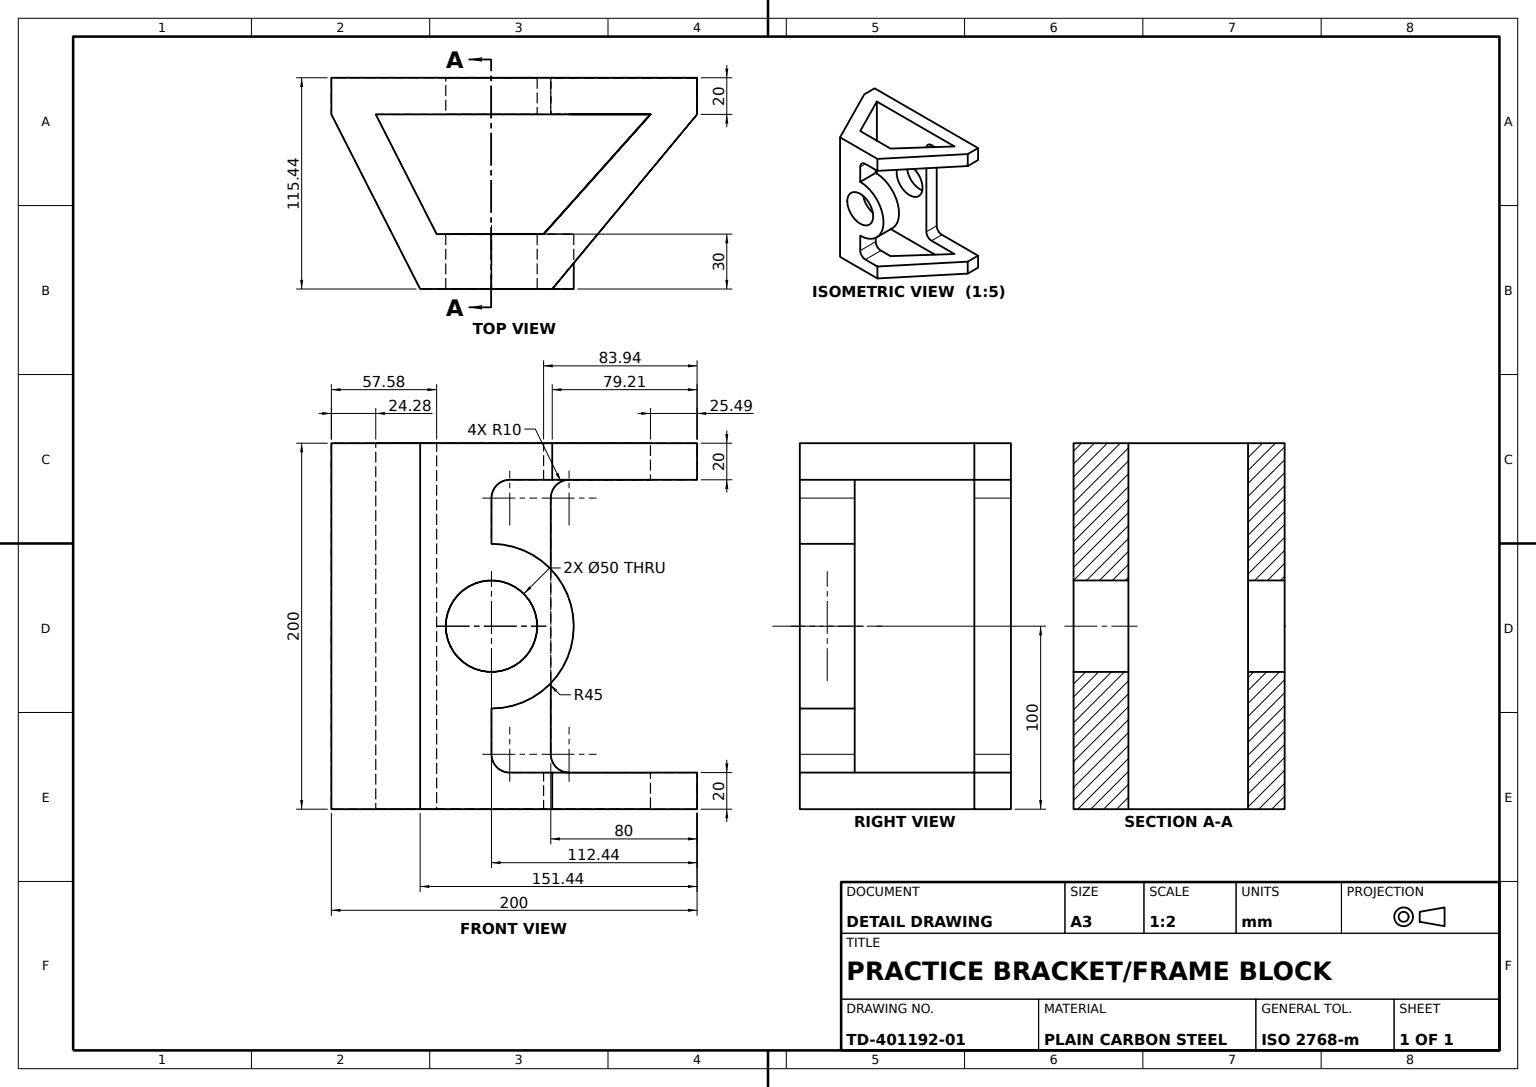
from build123d import *

# Parameters (mm, degrees)
BASE_PROFILE_20MM_DEPTH   = 20
A_FRAME_BODY_200MM_DEPTH  = 200
FRAME_WINDOW_1_SKETCH_W   = 124.025088206
FRAME_WINDOW_1_SKETCH_H   = 160
FRAME_WINDOW_1_CUT_DEPTH  = 30
FRAME_WINDOW_2_SKETCH_W   = 43.365918468
FRAME_WINDOW_2_SKETCH_H   = 160
FRAME_WINDOW_2_CUT_DEPTH  = 30
THROUGH_OPENING_SKETCH_W  = 51.957421724
THROUGH_OPENING_SKETCH_H  = 25.341390787
THROUGH_OPENING_CUT_DEPTH = 200
WEB_BOSS_30MM_DEPTH       = 30
HUB_BOSS_30MM_DEPTH       = 30
HUB_BORE_SKETCH_R         = 25
HUB_BORE_CUT_DEPTH        = 120


with BuildPart() as part:
    # Base Profile Sketch → Base Profile 20mm (new body)
    with BuildSketch(Plane.XY):
        with BuildLine():
            Line((0, 200), (0, 0))
            Line((0, 0), (200, 0))
            Line((200, 0), (200, 20))
            Line((200, 20), (130, 20))
            ThreePointArc((130, 20), (122.928932188, 22.928932188), (120, 30))
            Line((120, 30), (120, 160))
            Line((120, 160), (120, 170))
            ThreePointArc((120, 170), (122.928932188, 177.071067812), (130, 180))
            Line((130, 180), (200, 180))
            Line((200, 180), (200, 200))
            Line((200, 200), (0, 200))
        make_face()
    extrude(amount=BASE_PROFILE_20MM_DEPTH)

    # Frame Profile Sketch → A-Frame Body 200mm (add)
    with BuildSketch(Plane.XZ):
        Polygon((120.794177907, 115.439301395), (94.123171193, 115.439301395), (91.530156651, 115.439301395), (48.56020139, 115.439301395), (0, 20), (24.280100695, 20), (59.946420611, 90.097910608), (111.903842335, 90.097910608), (174.506621983, 20), (200, 20), align=None)
    extrude(amount=-A_FRAME_BODY_200MM_DEPTH)

    # Frame Window 1 Sketch → Frame Window 1 Cut (cut)
    with BuildSketch(Plane(origin=(128.259685241, 0, 106.443715141), x_dir=(0.6386274199814919, 0, -0.7695160936899132), z_dir=(0.7695160936899134, 0, 0.6386274199814919))):
        with Locations((50.32261802, 100)):
            Rectangle(FRAME_WINDOW_1_SKETCH_W, FRAME_WINDOW_1_SKETCH_H)
    extrude(amount=-FRAME_WINDOW_1_CUT_DEPTH, mode=Mode.SUBTRACT)

    # Frame Window 2 Sketch → Frame Window 2 Cut (cut)
    with BuildSketch(Plane.XY.offset(115.439301395)):
        with Locations((99.111218673, 100)):
            Rectangle(FRAME_WINDOW_2_SKETCH_W, FRAME_WINDOW_2_SKETCH_H)
    extrude(amount=-FRAME_WINDOW_2_CUT_DEPTH, mode=Mode.SUBTRACT)

    # Through Opening Sketch → Through Opening Cut (cut)
    with BuildSketch(Plane.XZ):
        with Locations((85.925131473, 102.768606002)):
            Rectangle(THROUGH_OPENING_SKETCH_W, THROUGH_OPENING_SKETCH_H)
    extrude(amount=-THROUGH_OPENING_CUT_DEPTH, mode=Mode.SUBTRACT)

    # Web Sketch → Web Boss 30mm (add)
    with BuildSketch(Plane.XY.offset(115.439301395)):
        with BuildLine():
            Line((48.56020139, 200), (120.794177907, 200))
            Line((120.794177907, 200), (120.794177907, 180))
            Line((120.794177907, 180), (97.556604563, 180))
            ThreePointArc((97.556604563, 180), (90.485536751, 177.071067812), (87.556604563, 170))
            Line((87.556604563, 170), (87.556604563, 30))
            ThreePointArc((87.556604563, 30), (90.485536751, 22.928932188), (97.556604563, 20))
            Line((97.556604563, 20), (120.794177907, 20))
            Line((120.794177907, 20), (120.794177907, 0))
            Line((120.794177907, 0), (48.56020139, 0))
            Line((48.56020139, 0), (48.56020139, 200))
        make_face()
    extrude(amount=-WEB_BOSS_30MM_DEPTH)

    # Hub Boss Sketch → Hub Boss 30mm (add)
    with BuildSketch(Plane.XY.offset(115.439301395)):
        with BuildLine():
            Line((87.556604563, 145), (87.556604563, 55))
            ThreePointArc((87.556604563, 55), (132.556604563, 100), (87.556604563, 145))
        make_face()
    extrude(amount=-HUB_BOSS_30MM_DEPTH)

    # Hub Bore Sketch → Hub Bore Cut (cut)
    with BuildSketch(Plane.XY.offset(115.439301395)):
        with Locations((87.556604563, 100)):
            Circle(HUB_BORE_SKETCH_R)
    extrude(amount=-HUB_BORE_CUT_DEPTH, mode=Mode.SUBTRACT)


solid = part.part
